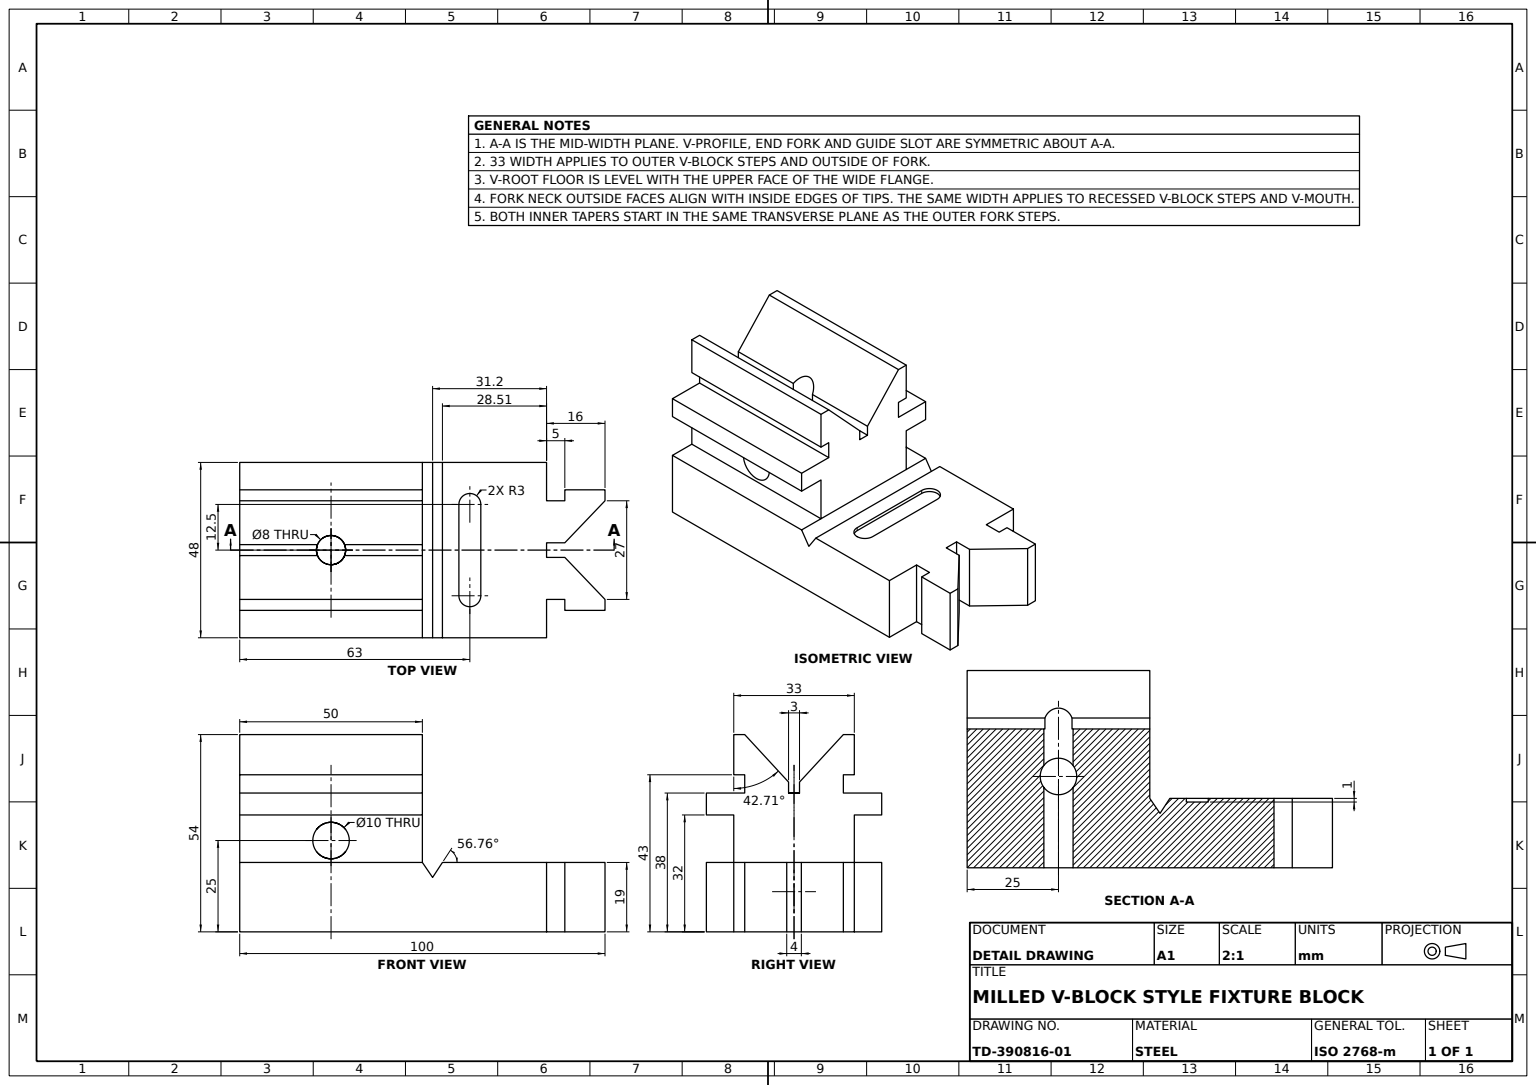
from build123d import *

# Parameters (mm, degrees)
BASE_BLOCK_PROFILE_W          = 100
BASE_BLOCK_PROFILE_H          = 19
BASE_BLOCK_100X19X48_DEPTH    = 24
END_NOTCHES_CUT_DEPTH         = 24
GUIDE_SLOT_63X3_DEPTH_1_DEPTH = 1
V_BLOCK_BODY_DEPTH            = 50
V_GROOVE_CUT_DEPTH            = 60
CROSS_HOLE_8_SKETCH_R         = 4
CROSS_HOLE_8_DEPTH            = 55
HOLE_10_SKETCH_R              = 5
HOLE_10_DEPTH                 = 60


with BuildPart() as part:
    # Base Block Profile → Base Block 100x19x48 (new, symmetric)
    with BuildSketch(Plane.XY):
        with Locations((50, 9.5)):
            Rectangle(BASE_BLOCK_PROFILE_W, BASE_BLOCK_PROFILE_H)
    extrude(amount=BASE_BLOCK_100X19X48_DEPTH, both=True)

    # End Notch Profile → End Notches Cut (cut, symmetric)
    with BuildSketch(Plane(origin=(0, 19, 0), x_dir=(1, 0, 0), z_dir=(0, 1, 0))):
        Polygon((100, -24), (100, -16.5), (89, -16.5), (89, -13.5), (84, -13.5), (84, -24), align=None)
        Polygon((100, -13.5), (100, 0), (84, 0), (84, -2), (89, -2), align=None)
        Polygon((100, 0), (100, 13.5), (89, 2), (84, 2), (84, 0), align=None)
        Polygon((100, 24), (84, 24), (84, 13.5), (89, 13.5), (89, 16.5), (100, 16.5), align=None)
    extrude(amount=END_NOTCHES_CUT_DEPTH, both=True, mode=Mode.SUBTRACT)

    # Guide Slot Sketch → Guide Slot 63x3 Depth 1 (cut)
    with BuildSketch(Plane(origin=(0, 19, 0), x_dir=(1, 0, 0), z_dir=(0, 1, 0))):
        with BuildLine():
            Line((60, -12.5), (60, 12.5))
            ThreePointArc((60, 12.5), (63, 15.5), (66, 12.5))
            Line((66, 12.5), (66, -12.5))
            ThreePointArc((66, -12.5), (63, -15.5), (60, -12.5))
        make_face()
    extrude(amount=-GUIDE_SLOT_63X3_DEPTH_1_DEPTH, mode=Mode.SUBTRACT)

    # V-Block Body Profile → V-Block Body (add)
    with BuildSketch(Plane.ZY):
        Polygon((-16.5, 19), (-16.5, 32), (-24, 32), (-24, 38), (-13.5, 38), (-13.5, 43), (-16.5, 43), (-16.5, 54), (-13.5, 54), (-1.5, 41), (-1.5, 38), (1.5, 38), (1.5, 41), (13.5, 54), (16.5, 54), (16.5, 43), (13.5, 43), (13.5, 38), (24, 38), (24, 32), (16.5, 32), (16.5, 19), align=None)
    extrude(amount=-V_BLOCK_BODY_DEPTH)

    # V-Groove Sketch → V-Groove Cut (cut)
    with BuildSketch(Plane.XY.offset(24)):
        Polygon((50, 19), (52.80194455, 14.895599546), (55.491811317, 19), align=None)
    extrude(amount=-V_GROOVE_CUT_DEPTH, mode=Mode.SUBTRACT)

    # Cross Hole Ø8 Sketch → Cross Hole Ø8 (cut, symmetric)
    with BuildSketch(Plane(origin=(0, 38, 0), x_dir=(1, 0, 0), z_dir=(0, 1, 0))):
        with Locations(Location((25, 0, 0), (0, 0, 270))):
            Circle(CROSS_HOLE_8_SKETCH_R)
    extrude(amount=CROSS_HOLE_8_DEPTH, both=True, mode=Mode.SUBTRACT)

    # Hole Ø10 Sketch → Hole Ø10 (cut)
    with BuildSketch(Plane.XY.offset(24)):
        with Locations(Location((25, 25, 0), (0, 0, 90))):
            Circle(HOLE_10_SKETCH_R)
    extrude(amount=-HOLE_10_DEPTH, mode=Mode.SUBTRACT)


solid = part.part
